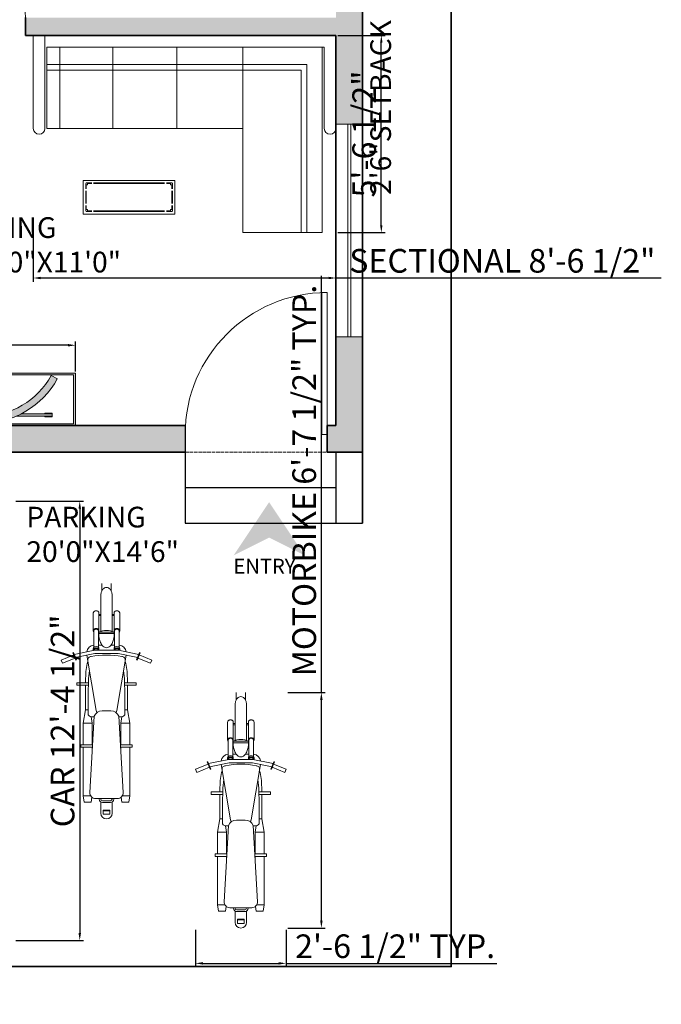
# Model space of a CAD drawing. Units: inches. Extents: x 4732 to 5926, y 2665 to 3255.
# Tile 5 of 8: x 5104 to 5321, y 2723 to 3056. Entities that reach past the tile are written whole.
import ezdxf

# ---------------------------------------------------------------- set-up
doc = ezdxf.new("R2010")
doc.units = ezdxf.units.IN
doc.linetypes.add('ACAD_ISO02W100', pattern=[15, 12, -3])
for name, color, linetype, lineweight in [('A-ANNO-DIMS', 2, 'Continuous', 18), ('A-ANNO-SYMB', 7, 'Continuous', 18), ('A-ANNO-TEXT', 7, 'Continuous', 18), ('A-AREA-IDEN', 7, 'Continuous', 18), ('A-DOOR', 3, 'Continuous', 18), ('A-FLOR-STRS', 7, 'Continuous', 25), ('A-FLOR-STRS-HIDN', 8, 'ACAD_ISO02W100', 18), ('A-GLAZ', 4, 'Continuous', 18), ('A-SITE-VEHS', 8, 'Continuous', 13), ('A-WALL', 7, 'Continuous', 35), ('A-WALL-PATT', 8, 'Continuous', 13), ('aparador', 36, 'Continuous', 9), ('C-PROP', 7, 'Continuous', 35), ('moveis', 254, 'Continuous', 5), ('NOI THAT', 42, 'Continuous', 18)]:
    doc.layers.add(name, color=color, linetype=linetype, lineweight=lineweight)
doc.styles.get("Standard").update_dxf_attribs({"font": 'arial.ttf'})
doc.dimstyles.new('ISO-25', dxfattribs={"dimtxt": 8, "dimasz": 2.5, "dimexe": 1.25, "dimexo": 0.625, "dimtad": 1, "dimdec": 1, "dimlunit": 3, "dimtxsty": 'Standard', "dimcen": 2.5, "dimadec": 0, "dimazin": 0, "dimtfac": 1, "dimtdec": 1, "dimtmove": 0, "dimatfit": 3, "dimfxl": 1, "dimarcsym": 0})

# ---------------------------------------------------------------- blocks, each defined once
blk = doc.blocks.new('TABLE-30A')
at = {"color": 0, "linetype": 'ByBlock'}
for p, q in [((0, 0), (0, 0.55)), ((0, 0.55), (1.5, 0.55)), ((0.051, 0.508), (0.042, 0.499)), ((0.042, 0.499), (0.042, 0.478)), ((0.072, 0.508), (0.051, 0.508)), ((0.072, 0.478), (0.072, 0.508)), ((0.072, 0.508), (0.14, 0.508)), ((0.072, 0.499), (0.14, 0.499)), ((1.331, 0.508), (0.169, 0.508)), ((1.331, 0.499), (0.169, 0.499)), ((1.428, 0.508), (1.36, 0.508)), ((1.428, 0.499), (1.36, 0.499)), ((1.428, 0.508), (1.428, 0.478)), ((1.449, 0.508), (1.428, 0.508)), ((1.458, 0.499), (1.449, 0.508)), ((1.458, 0.478), (1.458, 0.499)), ((1.5, 0.55), (1.5, 0)), ((0.042, 0.478), (0.072, 0.478)), ((0.042, 0.478), (0.042, 0.41)), ((0.042, 0.169), (0.042, 0.381)), ((0.051, 0.478), (0.051, 0.41)), ((0.051, 0.169), (0.051, 0.381)), ((1.428, 0.478), (1.458, 0.478)), ((1.449, 0.478), (1.449, 0.41)), ((1.449, 0.381), (1.449, 0.169)), ((1.458, 0.478), (1.458, 0.41)), ((1.458, 0.381), (1.458, 0.169)), ((1.5, 0), (0, 0)), ((0.042, 0.072), (0.042, 0.14)), ((0.042, 0.072), (0.042, 0.051)), ((0.072, 0.072), (0.042, 0.072)), ((0.042, 0.051), (0.051, 0.042)), ((0.051, 0.072), (0.051, 0.14)), ((0.051, 0.042), (0.072, 0.042)), ((0.072, 0.042), (0.072, 0.072)), ((0.072, 0.051), (0.14, 0.051)), ((0.072, 0.042), (0.14, 0.042)), ((0.169, 0.051), (1.331, 0.051)), ((0.169, 0.042), (1.331, 0.042)), ((1.428, 0.051), (1.36, 0.051)), ((1.428, 0.042), (1.36, 0.042)), ((1.428, 0.072), (1.428, 0.042)), ((1.458, 0.072), (1.428, 0.072)), ((1.428, 0.042), (1.449, 0.042)), ((1.449, 0.072), (1.449, 0.14)), ((1.449, 0.042), (1.458, 0.051)), ((1.458, 0.072), (1.458, 0.14)), ((1.458, 0.051), (1.458, 0.072))]:
    blk.add_line(p, q, dxfattribs=at)
blk = doc.blocks.new('12')
at = {"color": 0}
for p, q in [((5656.26, 3021.25), (5553.9, 3021.25)), ((5553.9, 3021.25), (5553.9, 2989.76)), ((5557.83, 3021.25), (5557.83, 2989.76)), ((5656.26, 2989.76), (5656.26, 3021.25)), ((5652.32, 3017.31), (5558.49, 3017.31)), ((5558.49, 3017.31), (5558.49, 2989.76)), ((5562.89, 3017.31), (5562.89, 2989.76)), ((5580.8, 3017.31), (5580.8, 2989.76)), ((5602.45, 3017.31), (5602.45, 2989.76)), ((5624.76, 3017.31), (5624.76, 2954.53)), ((5651.66, 3017.31), (5651.66, 2954.53)), ((5652.32, 2989.76), (5652.32, 3017.31)), ((5646.42, 3011.41), (5558.49, 3011.41)), ((5646.42, 2954.53), (5646.42, 3011.41)), ((5644.45, 3009.44), (5558.49, 3009.44)), ((5644.45, 2954.53), (5644.45, 3009.44)), ((5624.76, 2995), (5624.76, 2954.53)), ((5558.49, 2989.76), (5624.76, 2989.76)), ((5651.66, 2954.53), (5624.76, 2954.53))]:
    blk.add_line(p, q, dxfattribs=at)
for centre in [(5555.86, 2989.76), (5654.29, 2989.76)]:
    blk.add_arc(centre, 1.97, 180, 0, dxfattribs=at)
at = {"xscale": -20.70834898381633, "yscale": 20.70834898381633, "zscale": 20.70834898381633}
blk.add_blockref('TABLE-30A', (5601.8, 2960.82), dxfattribs=at)
blk = doc.blocks.new('Aparador ORGANICA Formatto')
at = {"layer": 'aparador', "ltscale": 0.3}
h = blk.add_hatch(color=256, dxfattribs=at)
h.dxf.hatch_style = 1
h.set_gradient(color1=(118, 213, 123), color2=(52, 168, 57), one_color=1, tint=0.43, name='INVCURVED')
h.paths.add_polyline_path([(0.8, 0.45), (-0.8, 0.45), (-0.8, 0), (0.8, 0)])
h.paths.add_polyline_path([(0.785, 0.435), (0.785, 0.015), (-0.785, 0.015), (-0.785, 0.435)], flags=16)
h.paths.add_polyline_path([(0.2911, 0.3699), (0.5365, 0.3699), (0.5365, 0.3757), (0.6011, 0.3757), (0.6011, 0.3699), (0.6011, 0.3499), (0.6011, 0.3441), (0.5365, 0.3441), (0.5365, 0.3499), (0.3338, 0.3499, -0.150336), (0.6449, 0.0488), (0.5923, 0.0199, 0.208852), (0.1632, 0.3499), (-0.1632, 0.3499, 0.208852), (-0.5923, 0.0199), (-0.6449, 0.0488, -0.150336), (-0.3338, 0.3499), (-0.5365, 0.3499), (-0.5365, 0.3441), (-0.6011, 0.3441), (-0.6011, 0.3499), (-0.6011, 0.3699), (-0.6011, 0.3757), (-0.5365, 0.3757), (-0.5365, 0.3699), (-0.2911, 0.3699, -0.206106)], flags=0)
h = blk.add_hatch(color=256, dxfattribs=at)
h.dxf.hatch_style = 1
h.set_gradient(color1=(135, 92, 69), color2=(0, 0, 0), one_color=1, name='INVCURVED')
h.paths.add_polyline_path([(-0.6449, 0.0488), (-0.5923, 0.0199, -0.590888), (0.5923, 0.0199), (0.6449, 0.0488, 0.590888)])
h = blk.add_hatch(color=256, dxfattribs=at)
h.dxf.hatch_style = 1
h.set_gradient(color1=(178, 189, 189), one_color=1, tint=1, name='CYLINDER')
h.paths.add_polyline_path([(-0.5365, 0.3757), (-0.6011, 0.3757), (-0.6011, 0.3699), (-0.5365, 0.3699)])
h.paths.add_polyline_path([(-0.5365, 0.3499), (-0.6011, 0.3499), (-0.6011, 0.3441), (-0.5365, 0.3441)])
h = blk.add_hatch(color=256, dxfattribs=at)
h.dxf.hatch_style = 1
h.set_gradient(color1=(118, 213, 123), color2=(31, 101, 35), one_color=1, tint=0.26, name='INVCURVED')
h.paths.add_polyline_path([(-0.2911, 0.3699), (-0.6011, 0.3699), (-0.6011, 0.3499), (-0.3338, 0.3499, -0.015999)])
h = blk.add_hatch(color=256, dxfattribs=at)
h.dxf.hatch_style = 1
h.set_gradient(color1=(118, 213, 123), color2=(31, 101, 35), one_color=1, tint=0.26, name='INVCURVED')
h.paths.add_polyline_path([(-0.1632, 0.3499), (0.1632, 0.3499, 0.122516)])
h = blk.add_hatch(color=256, dxfattribs=at)
h.dxf.hatch_style = 1
h.set_gradient(color1=(118, 213, 123), color2=(31, 101, 35), one_color=1, tint=0.26, name='INVCURVED')
h.paths.add_polyline_path([(0.6011, 0.3699), (0.2911, 0.3699, -0.015999), (0.3338, 0.3499), (0.6011, 0.3499)])
h = blk.add_hatch(color=256, dxfattribs=at)
h.dxf.hatch_style = 1
h.set_gradient(color1=(178, 189, 189), one_color=1, tint=1, name='CYLINDER')
h.paths.add_polyline_path([(0.6011, 0.3757), (0.5365, 0.3757), (0.5365, 0.3699), (0.6011, 0.3699)])
h.paths.add_polyline_path([(0.6011, 0.3499), (0.5365, 0.3499), (0.5365, 0.3441), (0.6011, 0.3441)])
for p, q in [((-0.5923, 0.0199), (-0.6449, 0.0488)), ((0.5923, 0.0199), (0.6449, 0.0488))]:
    blk.add_line(p, q, dxfattribs=at)
for points in [[(-0.6011, 0.3699), (-0.6011, 0.3757), (-0.5365, 0.3757), (-0.5365, 0.3699)], [(-0.5365, 0.3499), (-0.5365, 0.3441), (-0.6011, 0.3441), (-0.6011, 0.3499)], [(0.6011, 0.3699), (0.6011, 0.3757), (0.5365, 0.3757), (0.5365, 0.3699)], [(0.5365, 0.3499), (0.5365, 0.3441), (0.6011, 0.3441), (0.6011, 0.3499)]]:
    blk.add_lwpolyline(points, dxfattribs=at)
for radius in [0.7362, 0.6762]:
    blk.add_arc((0, -0.3063), radius, 28.84335, 151.15665, dxfattribs=at)
at = {"layer": 'moveis', "ltscale": 0.3}
for p, q in [((-0.6011, 0.3699), (-0.6011, 0.3499)), ((-0.2911, 0.3699), (-0.6011, 0.3699)), ((-0.6011, 0.3499), (-0.3338, 0.3499)), ((-0.1632, 0.3499), (0.1632, 0.3499)), ((0.2911, 0.3699), (0.6011, 0.3699)), ((0.6011, 0.3499), (0.3338, 0.3499)), ((0.6011, 0.3699), (0.6011, 0.3499))]:
    blk.add_line(p, q, dxfattribs=at)
for points in [[(-0.8, 0), (0.8, 0), (0.8, 0.45), (-0.8, 0.45)], [(-0.785, 0.015), (0.785, 0.015), (0.785, 0.435), (-0.785, 0.435)]]:
    blk.add_lwpolyline(points, close=True, dxfattribs=at)
blk = doc.blocks.new('*U20')
for p, q in [((0, 0), (0, -6)), ((36, 0), (36, -6))]:
    blk.add_line(p, q)
blk.add_lwpolyline([(0, 0), (0, 36), (1.75, 36), (1.75, 0)], close=True)
blk.add_arc((0, 0), 36, 0, 90)
blk = doc.blocks.new('BIKE')
for p, q in [((34846.04, 15170.34), (34846.04, 15168.87)), ((34847.86, 15170.34), (34847.86, 15168.87)), ((34845.81, 15167.86), (34845.81, 15160.7)), ((34845.81, 15167.86), (34845.81, 15160.7)), ((34848.09, 15167.86), (34848.09, 15160.7)), ((34844.29, 15164.4), (34844.29, 15160.81)), ((34845.43, 15164.4), (34845.43, 15160.81)), ((34845.43, 15164.1), (34845.81, 15164.1)), ((34845.43, 15163.85), (34845.81, 15163.85)), ((34848.47, 15164.1), (34848.09, 15164.1)), ((34848.47, 15163.85), (34848.09, 15163.85)), ((34848.47, 15164.4), (34848.47, 15160.81)), ((34849.61, 15164.4), (34849.61, 15160.81)), ((34844.41, 15160.81), (34844.41, 15157.43)), ((34845.32, 15160.81), (34845.32, 15157.43)), ((34848.51, 15160.53), (34845.39, 15160.53)), ((34845.39, 15160.23), (34845.39, 15160.53)), ((34845.39, 15160.23), (34845.39, 15160.53)), ((34848.51, 15160.23), (34845.39, 15160.23)), ((34848.51, 15160.23), (34848.51, 15160.53)), ((34848.58, 15160.81), (34848.58, 15157.43)), ((34849.5, 15160.81), (34849.5, 15157.43)), ((34845.32, 15157.92), (34846.04, 15157.92)), ((34848.58, 15157.92), (34847.87, 15157.92)), ((34837.84, 15154.89), (34840.37, 15155.93)), ((34840.19, 15156.35), (34840.3, 15156.39)), ((34840.19, 15156.35), (34840.8, 15154.88)), ((34840.3, 15156.39), (34840.9, 15154.92)), ((34840.47, 15155.97), (34840.8, 15156.11)), ((34840.8, 15156.11), (34844.56, 15156.88)), ((34841, 15155.45), (34844.63, 15156.2)), ((34844.86, 15144.72), (34843.01, 15155.87)), ((34844.29, 15156.87), (34844.29, 15157.17)), ((34844.41, 15156.87), (34844.41, 15156.85)), ((34844.56, 15156.88), (34846.95, 15156.88)), ((34844.63, 15156.2), (34846.95, 15156.2)), ((34845.43, 15156.87), (34845.43, 15157.17)), ((34849.34, 15156.88), (34846.95, 15156.88)), ((34849.27, 15156.2), (34846.95, 15156.2)), ((34848.47, 15156.87), (34848.47, 15157.17)), ((34849.05, 15144.72), (34850.89, 15155.87)), ((34852.9, 15155.45), (34849.27, 15156.2)), ((34853.1, 15156.11), (34849.34, 15156.88)), ((34849.5, 15156.87), (34849.5, 15156.85)), ((34849.61, 15156.87), (34849.61, 15157.17)), ((34853.6, 15156.39), (34853, 15154.92)), ((34853.71, 15156.35), (34853.1, 15154.88)), ((34853.43, 15155.97), (34853.1, 15156.11)), ((34856.07, 15154.89), (34853.54, 15155.93)), ((34853.71, 15156.35), (34853.6, 15156.39)), ((34837.84, 15154.89), (34838.1, 15154.26)), ((34838.1, 15154.26), (34840.63, 15155.3)), ((34840.73, 15155.34), (34841, 15155.45)), ((34840.8, 15154.88), (34840.9, 15154.92)), ((34842.8, 15152.59), (34843.06, 15154.2)), ((34843.06, 15154.2), (34843.22, 15154.58)), ((34850.84, 15154.2), (34850.68, 15154.58)), ((34851.1, 15152.59), (34850.84, 15154.2)), ((34853.17, 15155.34), (34852.9, 15155.45)), ((34853.1, 15154.88), (34853, 15154.92)), ((34855.81, 15154.26), (34853.28, 15155.3)), ((34856.07, 15154.89), (34855.81, 15154.26)), ((34842.7, 15150.31), (34842.8, 15152.59)), ((34843.33, 15151.09), (34843.52, 15152.8)), ((34850.57, 15151.09), (34850.38, 15152.8)), ((34851.2, 15150.31), (34851.1, 15152.59)), ((34840.97, 15150.31), (34843.3, 15150.31)), ((34840.97, 15149.81), (34840.97, 15150.31)), ((34843.29, 15149.81), (34840.97, 15149.81)), ((34842.7, 15144.87), (34842.7, 15149.81)), ((34843.23, 15147.75), (34843.33, 15151.09)), ((34850.67, 15147.75), (34850.57, 15151.09)), ((34852.93, 15150.31), (34850.6, 15150.31)), ((34850.61, 15149.81), (34852.93, 15149.81)), ((34851.2, 15144.87), (34851.2, 15149.81)), ((34852.93, 15149.81), (34852.93, 15150.31)), ((34843.23, 15144.15), (34843.23, 15147.75)), ((34850.67, 15144.15), (34850.67, 15147.75)), ((34842.7, 15144.87), (34842.25, 15142.19)), ((34842.7, 15144.87), (34843.23, 15144.87)), ((34847.85, 15144.64), (34846.06, 15144.64)), ((34851.2, 15144.87), (34850.67, 15144.87)), ((34851.2, 15144.87), (34851.65, 15142.19)), ((34842.25, 15142.19), (34844.07, 15142.19)), ((34842.25, 15137.82), (34842.25, 15142.19)), ((34844.46, 15143.56), (34843.6, 15128.2)), ((34843.85, 15143.46), (34844.07, 15142.19)), ((34843.91, 15143.46), (34844.46, 15143.46)), ((34844.07, 15137.82), (34844.07, 15142.19)), ((34849.44, 15143.56), (34850.3, 15128.2)), ((34849.99, 15143.46), (34849.44, 15143.46)), ((34850.05, 15143.46), (34849.83, 15142.19)), ((34851.65, 15142.19), (34849.83, 15142.19)), ((34849.83, 15137.82), (34849.83, 15142.19)), ((34851.65, 15137.82), (34851.65, 15142.19)), ((34841.79, 15137.82), (34844.14, 15137.82)), ((34841.79, 15137.33), (34841.79, 15137.82)), ((34844.11, 15137.33), (34841.79, 15137.33)), ((34842.25, 15127.57), (34842.25, 15137.33)), ((34844.07, 15136.55), (34844.07, 15137.33)), ((34852.11, 15137.82), (34849.76, 15137.82)), ((34849.79, 15137.33), (34852.11, 15137.33)), ((34849.83, 15136.55), (34849.83, 15137.33)), ((34851.65, 15127.57), (34851.65, 15137.33)), ((34852.11, 15137.33), (34852.11, 15137.82)), ((34842.25, 15127.57), (34843.75, 15127.57)), ((34842.25, 15127.57), (34842.48, 15126.27)), ((34842.48, 15126.27), (34843.84, 15126.27)), ((34844.02, 15127.25), (34843.84, 15126.27)), ((34849.16, 15126.99), (34844.74, 15126.99)), ((34845.47, 15126.99), (34845.47, 15126.88)), ((34845.81, 15126.99), (34845.81, 15126.88)), ((34845.81, 15126.29), (34845.81, 15124.03)), ((34847.75, 15126.54), (34846.15, 15126.54)), ((34847.75, 15126.2), (34846.15, 15126.2)), ((34848.09, 15126.99), (34848.09, 15126.88)), ((34848.09, 15126.29), (34848.09, 15124.03)), ((34848.43, 15126.99), (34848.43, 15126.88)), ((34849.89, 15127.25), (34850.06, 15126.27)), ((34851.43, 15126.27), (34850.06, 15126.27)), ((34851.65, 15127.57), (34850.15, 15127.57)), ((34851.65, 15127.57), (34851.43, 15126.27)), ((34846.29, 15123.82), (34846.29, 15124.66)), ((34846.29, 15124.66), (34847.61, 15124.66)), ((34846.29, 15124.55), (34847.61, 15124.55)), ((34847.61, 15124.66), (34847.61, 15123.82)), ((34847.61, 15123.82), (34846.29, 15123.82))]:
    blk.add_line(p, q)
for points in [[(34845.81, 15167.86, -0.068977), (34845.9, 15168.53, -0.081012), (34846.15, 15169.05, -0.107014), (34846.54, 15169.42, -0.137239), (34846.95, 15169.53, -0.137239), (34847.36, 15169.42, -0.107014), (34847.76, 15169.05, -0.081012), (34848, 15168.53, -0.068977), (34848.09, 15167.86, -0.068977)], [(34845.43, 15164.4, 0.125099), (34845.39, 15164.56, 0.105827), (34845.27, 15164.71, 0.086577), (34845.09, 15164.8, 0.0766), (34844.86, 15164.84, 0.0766), (34844.64, 15164.8, 0.086577), (34844.46, 15164.71, 0.105827), (34844.33, 15164.56, 0.125099), (34844.29, 15164.4, 0.125099)], [(34848.47, 15164.4, -0.125099), (34848.51, 15164.56, -0.105827), (34848.64, 15164.71, -0.086577), (34848.82, 15164.8, -0.0766), (34849.04, 15164.84, -0.0766), (34849.26, 15164.8, -0.086577), (34849.44, 15164.71, -0.105827), (34849.57, 15164.56, -0.125099), (34849.61, 15164.4, -0.125099)], [(34845.32, 15160.55, 0.067261), (34845.39, 15160.65, 0.125099), (34845.43, 15160.81, 0.125099), (34845.39, 15160.97, 0.105827), (34845.27, 15161.12, 0.086577), (34845.09, 15161.21, 0.0766), (34844.86, 15161.25, 0.0766), (34844.64, 15161.21, 0.086577), (34844.46, 15161.12, 0.105827), (34844.33, 15160.97, 0.125099), (34844.29, 15160.81, 0.125099)], [(34844.29, 15160.81, 0.125099), (34844.33, 15160.65, 0.067261), (34844.41, 15160.55, 0.086577)], [(34845.32, 15160.81, 0.125099), (34845.29, 15160.92, 0.105827), (34845.2, 15161.03, 0.086577), (34845.05, 15161.1, 0.0766), (34844.86, 15161.13, 0.0766), (34844.67, 15161.1, 0.086577), (34844.53, 15161.03, 0.105827), (34844.43, 15160.92, 0.125099), (34844.41, 15160.81, 0.125099)], [(34846.95, 15157.37, -0.163989), (34846.41, 15157.55, -0.105862), (34845.85, 15158.21, -0.069323), (34845.52, 15159.08, -0.055531), (34845.39, 15160.23, -0.055531)], [(34848.51, 15160.23, -0.055531), (34848.38, 15159.08, -0.069323), (34848.06, 15158.21, -0.105862), (34847.49, 15157.55, -0.163989), (34846.95, 15157.37, -0.163989)], [(34848.58, 15160.55, -0.067261), (34848.51, 15160.65, -0.125099), (34848.47, 15160.81, -0.125099), (34848.51, 15160.97, -0.105827), (34848.64, 15161.12, -0.086577), (34848.82, 15161.21, -0.0766), (34849.04, 15161.25, -0.0766), (34849.26, 15161.21, -0.086577), (34849.44, 15161.12, -0.105827), (34849.57, 15160.97, -0.125099), (34849.61, 15160.81, -0.125099)], [(34848.58, 15160.81, -0.125099), (34848.61, 15160.92, -0.105827), (34848.71, 15161.03, -0.086577), (34848.85, 15161.1, -0.0766), (34849.04, 15161.13, -0.0766), (34849.23, 15161.1, -0.086577), (34849.37, 15161.03, -0.105827), (34849.47, 15160.92, -0.125099), (34849.5, 15160.81, -0.125099)], [(34849.61, 15160.81, -0.125099), (34849.57, 15160.65, -0.067261), (34849.5, 15160.55, -0.086577)], [(34845.43, 15157.17, 0.125099), (34845.39, 15157.33, 0.105827), (34845.27, 15157.48, 0.086577), (34845.09, 15157.57, 0.0766), (34844.86, 15157.6, 0.0766), (34844.64, 15157.57, 0.086577), (34844.46, 15157.48, 0.105827), (34844.33, 15157.33, 0.125099), (34844.29, 15157.17, 0.125099)], [(34845.43, 15156.88, 0.117252), (34845.39, 15157.03, 0.105827), (34845.27, 15157.18, 0.086577), (34845.09, 15157.27, 0.0766), (34844.86, 15157.31, 0.0766), (34844.64, 15157.27, 0.086577), (34844.46, 15157.18, 0.105827), (34844.33, 15157.03, 0.125099), (34844.29, 15156.87, 0.125099)], [(34844.29, 15156.87, 0.032819), (34844.3, 15156.83, 0.067261)], [(34845.32, 15156.88, 0.113202), (34845.29, 15156.98, 0.105827), (34845.2, 15157.09, 0.086577), (34845.05, 15157.16, 0.0766), (34844.86, 15157.19, 0.0766), (34844.67, 15157.16, 0.086577), (34844.53, 15157.09, 0.105827), (34844.43, 15156.98, 0.125099), (34844.41, 15156.87, 0.125099)], [(34848.47, 15157.17, -0.125099), (34848.51, 15157.33, -0.105827), (34848.64, 15157.48, -0.086577), (34848.82, 15157.57, -0.0766), (34849.04, 15157.6, -0.0766), (34849.26, 15157.57, -0.086577), (34849.44, 15157.48, -0.105827), (34849.57, 15157.33, -0.125099), (34849.61, 15157.17, -0.125099)], [(34848.47, 15156.88, -0.117252), (34848.51, 15157.03, -0.105827), (34848.64, 15157.18, -0.086577), (34848.82, 15157.27, -0.0766), (34849.04, 15157.31, -0.0766), (34849.26, 15157.27, -0.086577), (34849.44, 15157.18, -0.105827), (34849.57, 15157.03, -0.125099), (34849.61, 15156.87, -0.125099)], [(34848.58, 15156.88, -0.113202), (34848.61, 15156.98, -0.105827), (34848.71, 15157.09, -0.086577), (34848.85, 15157.16, -0.0766), (34849.04, 15157.19, -0.0766), (34849.23, 15157.16, -0.086577), (34849.37, 15157.09, -0.105827), (34849.47, 15156.98, -0.125099), (34849.5, 15156.87, -0.125099)], [(34849.61, 15156.87, -0.032819), (34849.61, 15156.83, -0.067261)]]:
    blk.add_lwpolyline(points, format="xyb")
for centre, radius, start, end in [((34846.95, 15157.24), 3.64, 64.5882, 115.4118), ((34844.55, 15156.32), 1.59, 95.2207, 171.678), ((34849.35, 15156.32), 1.59, 8.322, 84.7793), ((34846.95, 15140.12), 15.79, 78.7129, 101.2871), ((34843.86, 15154.92), 0.684, 90, 189.3898), ((34850.04, 15154.92), 0.684, 350.6102, 90), ((34843.91, 15144.15), 0.684, 180, 270), ((34846, 15143), 1.64, 88.1125, 159.9264), ((34845.53, 15144.83), 0.684, 189.3898, 226.4877), ((34847.9, 15143), 1.64, 20.0736, 91.8875), ((34848.37, 15144.83), 0.684, 313.5123, 350.6102), ((34849.99, 15144.15), 0.684, 270, 0), ((34844.74, 15128.13), 1.14, 176.7865, 270), ((34849.16, 15128.13), 1.14, 270, 3.2135), ((34846.15, 15126.88), 0.684, 180, 270), ((34846.15, 15126.88), 0.342, 180, 270), ((34847.75, 15126.88), 0.684, 270, 0), ((34847.75, 15126.88), 0.342, 270, 0), ((34846.95, 15124.03), 1.14, 180, 0)]:
    blk.add_arc(centre, radius, start, end)
blk = doc.blocks.new('GLAZ-UNIT-72IN')
for p, q in [((0, 72), (0, 0)), ((1, 72), (1, 0))]:
    blk.add_line(p, q)
blk = doc.blocks.new('*D80')
at = {"layer": 'A-ANNO-DIMS', "color": 0, "lineweight": -2, "transparency": 16777216}
for p, q in [((5206.46, 2828.61), (5206.46, 2969.57)), ((5195.13, 2828.61), (5207.71, 2828.61)), ((5206.46, 2751.44), (5206.46, 2826.11)), ((5195.13, 2748.94), (5207.71, 2748.94))]:
    blk.add_line(p, q, dxfattribs=at)
at = {"layer": 'A-ANNO-DIMS', "color": 0, "transparency": 16777216}
for points in [[(5206.04, 2826.11), (5206.87, 2826.11), (5206.46, 2828.61)], [(5206.04, 2751.44), (5206.87, 2751.44), (5206.46, 2748.94)]]:
    blk.add_solid(points, dxfattribs=at)
at = {"layer": 'Defpoints', "color": 0, "transparency": 16777216}
for p in [(5194.51, 2828.61), (5206.46, 2828.61), (5194.51, 2748.94)]:
    blk.add_point(p, dxfattribs=at)
at = {"layer": 'A-ANNO-DIMS', "color": 0, "transparency": 16777216, "insert": (5201.69, 2900.34), "char_height": 8, "attachment_point": 5, "rotation": 90}
blk.add_mtext('MOTORBIKE 6\'-7 1/2" TYP.', dxfattribs=at)
blk = doc.blocks.new('*D81')
at = {"layer": 'A-ANNO-DIMS', "color": 0, "lineweight": -2, "transparency": 16777216}
for p, q in [((5163.91, 2748.32), (5163.91, 2735.74)), ((5194.51, 2748.32), (5194.51, 2735.74)), ((5166.41, 2736.99), (5192.01, 2736.99)), ((5194.51, 2736.99), (5265.8, 2736.99))]:
    blk.add_line(p, q, dxfattribs=at)
at = {"layer": 'A-ANNO-DIMS', "color": 0, "transparency": 16777216}
for points in [[(5166.41, 2737.41), (5166.41, 2736.57), (5163.91, 2736.99)], [(5192.01, 2737.41), (5192.01, 2736.57), (5194.51, 2736.99)]]:
    blk.add_solid(points, dxfattribs=at)
at = {"layer": 'Defpoints', "color": 0, "transparency": 16777216}
for p in [(5163.91, 2748.94), (5194.51, 2748.94), (5194.51, 2736.99)]:
    blk.add_point(p, dxfattribs=at)
at = {"layer": 'A-ANNO-DIMS', "color": 0, "transparency": 16777216, "insert": (5231.4, 2741.75), "char_height": 8, "attachment_point": 5}
blk.add_mtext('2\'-6 1/2" TYP.', dxfattribs=at)
blk = doc.blocks.new('*D92')
at = {"layer": 'A-ANNO-DIMS', "color": 0, "lineweight": -2, "transparency": 16777216}
for p, q in [((5109.02, 2983.58), (5109.02, 2967.6)), ((5211.38, 2983.58), (5211.38, 2967.6)), ((5111.52, 2968.85), (5208.88, 2968.85)), ((5211.38, 2968.85), (5321.45, 2968.85))]:
    blk.add_line(p, q, dxfattribs=at)
at = {"layer": 'A-ANNO-DIMS', "color": 0, "transparency": 16777216}
for points in [[(5111.52, 2969.27), (5111.52, 2968.44), (5109.02, 2968.85)], [(5208.88, 2969.27), (5208.88, 2968.44), (5211.38, 2968.85)]]:
    blk.add_solid(points, dxfattribs=at)
at = {"layer": 'Defpoints', "color": 0, "transparency": 16777216}
for p in [(5109.02, 2984.21), (5211.38, 2984.21), (5211.38, 2968.85)]:
    blk.add_point(p, dxfattribs=at)
at = {"layer": 'A-ANNO-DIMS', "color": 0, "transparency": 16777216, "insert": (5267.67, 2973.62), "char_height": 8, "attachment_point": 5}
blk.add_mtext('SECTIONAL 8\'-6 1/2"', dxfattribs=at)
blk = doc.blocks.new('*D93')
at = {"layer": 'A-ANNO-DIMS', "color": 0, "lineweight": -2, "transparency": 16777216}
for p, q in [((5212.01, 3050.93), (5227.99, 3050.93)), ((5226.74, 2986.71), (5226.74, 3048.43)), ((5212.01, 2984.21), (5227.99, 2984.21))]:
    blk.add_line(p, q, dxfattribs=at)
at = {"layer": 'A-ANNO-DIMS', "color": 0, "transparency": 16777216}
for points in [[(5226.32, 3048.43), (5227.15, 3048.43), (5226.74, 3050.93)], [(5226.32, 2986.71), (5227.15, 2986.71), (5226.74, 2984.21)]]:
    blk.add_solid(points, dxfattribs=at)
at = {"layer": 'Defpoints', "color": 0, "transparency": 16777216}
for p in [(5211.38, 3050.93), (5226.74, 3050.93), (5211.38, 2984.21)]:
    blk.add_point(p, dxfattribs=at)
at = {"layer": 'A-ANNO-DIMS', "color": 0, "transparency": 16777216, "insert": (5221.97, 3017.57), "char_height": 8, "attachment_point": 5, "rotation": 90}
blk.add_mtext('5\'-6 1/2"', dxfattribs=at)
blk = doc.blocks.new('*D94')
at = {"layer": 'A-ANNO-DIMS', "color": 0, "lineweight": -2, "transparency": 16777216}
for p, q in [((5060.26, 2946.1), (4966.35, 2946.1)), ((5060.26, 2937.27), (5060.26, 2947.35)), ((5120.75, 2946.1), (5062.76, 2946.1)), ((5123.25, 2937.27), (5123.25, 2947.35))]:
    blk.add_line(p, q, dxfattribs=at)
at = {"layer": 'A-ANNO-DIMS', "color": 0, "transparency": 16777216}
for points in [[(5062.76, 2946.52), (5062.76, 2945.68), (5060.26, 2946.1)], [(5120.75, 2946.52), (5120.75, 2945.68), (5123.25, 2946.1)]]:
    blk.add_solid(points, dxfattribs=at)
at = {"layer": 'Defpoints', "color": 0, "transparency": 16777216}
for p in [(5060.26, 2946.1), (5060.26, 2936.65), (5123.25, 2936.65)]:
    blk.add_point(p, dxfattribs=at)
at = {"layer": 'A-ANNO-DIMS', "color": 0, "transparency": 16777216, "insert": (5012.05, 2950.87), "char_height": 8, "attachment_point": 5}
blk.add_mtext('SIDEBOARD 5\'-3"', dxfattribs=at)
blk = doc.blocks.new('*D96')
at = {"layer": 'A-ANNO-DIMS', "color": 0, "lineweight": -2, "transparency": 16777216}
for p, q in [((5103.06, 2893.31), (5125.97, 2893.31)), ((5124.72, 2890.81), (5124.72, 2747.23)), ((5103.06, 2744.73), (5125.97, 2744.73))]:
    blk.add_line(p, q, dxfattribs=at)
at = {"layer": 'A-ANNO-DIMS', "color": 0, "transparency": 16777216}
for points in [[(5124.3, 2890.81), (5125.14, 2890.81), (5124.72, 2893.31)], [(5124.3, 2747.23), (5125.14, 2747.23), (5124.72, 2744.73)]]:
    blk.add_solid(points, dxfattribs=at)
at = {"layer": 'Defpoints', "color": 0, "transparency": 16777216}
for p in [(5102.43, 2893.31), (5102.43, 2744.73), (5124.72, 2744.73)]:
    blk.add_point(p, dxfattribs=at)
at = {"layer": 'A-ANNO-DIMS', "color": 0, "transparency": 16777216, "insert": (5119.96, 2819.02), "char_height": 8, "attachment_point": 5, "rotation": 90}
blk.add_mtext('CAR 12\'-4 1/2"', dxfattribs=at)

msp = doc.modelspace()

# ---------------------------------------------------------------- hatches: boundary and pattern name
at = {"layer": 'A-ANNO-SYMB'}
h = msp.add_hatch(color=256, dxfattribs=at)
h.dxf.hatch_style = 1
h.paths.add_polyline_path([(5188.79, 2881.01), (5200.79, 2875.01), (5188.79, 2893.01), (5176.79, 2875.01)])
at = {"layer": 'A-WALL-PATT'}
h = msp.add_hatch(color=256, dxfattribs=at)
h.dxf.hatch_style = 1
h.paths.add_polyline_path([(4905.38, 3185.93), (4848.38, 3185.93), (4848.38, 3146.93), (4857.38, 3146.93), (4857.38, 3176.93), (4905.38, 3176.93)])
h.paths.add_polyline_path([(5022.38, 3185.93), (4953.38, 3185.93), (4953.38, 3176.93), (4966.1, 3176.93), (5001.38, 3176.93), (5001.38, 3098.93), (5028.38, 3098.93), (5028.38, 3104.93), (5007.38, 3104.93), (5007.38, 3176.93), (5022.38, 3176.93)])
h.paths.add_polyline_path([(5115.38, 3185.93), (5046.38, 3185.93), (5046.38, 3176.93), (5061.38, 3176.93), (5061.38, 3104.93), (5058.38, 3104.93), (5058.38, 3098.93), (5067.38, 3098.93), (5067.38, 3176.93), (5115.38, 3176.93)])
h.paths.add_polyline_path([(5220.38, 3185.93), (5163.38, 3185.93), (5163.38, 3176.93), (5168.97, 3176.93), (5211.38, 3176.93), (5211.38, 3146.93), (5220.38, 3146.93)])
h.paths.add_polyline_path([(4857.38, 3086.93), (4848.38, 3086.93), (4848.38, 3026.93), (4857.38, 3026.93), (4857.38, 3050.93), (5001.38, 3050.93), (5001.38, 3008.93), (5007.38, 3008.93), (5007.38, 3050.93), (5022.38, 3050.93), (5022.38, 3056.93), (4857.38, 3056.93)])
h.paths.add_polyline_path([(4857.38, 2978.93), (4848.38, 2978.93), (4848.38, 2945.93), (4872.38, 2945.93), (4872.38, 2933.93), (4875.38, 2933.93), (4881.38, 2933.93), (4881.38, 2954.93), (4857.38, 2954.93)])
h.paths.add_polyline_path([(4881.38, 2903.93), (4875.38, 2903.93), (4872.38, 2903.93), (4872.38, 2897.93), (4881.38, 2897.93)])
h.paths.add_polyline_path([(4881.38, 2849.93), (4872.38, 2849.93), (4872.38, 2828.75), (4872.38, 2825.93), (4848.38, 2825.93), (4848.38, 2804.93), (4857.38, 2804.93), (4857.38, 2816.93), (4929.38, 2816.93), (4929.38, 2825.93), (4881.38, 2825.93)])
h.paths.add_polyline_path([(4975.38, 2744.93), (4857.38, 2744.93), (4857.38, 2756.93), (4848.38, 2756.93), (4848.38, 2735.93), (4975.38, 2735.93)])
h.paths.add_polyline_path([(5160.38, 2915.93), (5160.38, 2918.93), (5007.38, 2918.93), (5007.38, 2960.93), (5001.38, 2960.93), (5001.38, 2825.93), (4977.38, 2825.93), (4977.38, 2816.93), (5010.38, 2816.93), (5010.38, 2909.93), (5160.38, 2909.93)])
h.paths.add_polyline_path([(5220.38, 2948.93), (5211.38, 2948.93), (5211.38, 2918.93), (5208.38, 2918.93), (5208.38, 2909.93), (5220.38, 2909.93)])
h.paths.add_polyline_path([(5220.38, 3086.93), (5211.38, 3086.93), (5211.38, 3056.93), (5106.38, 3056.93), (5106.38, 3050.93), (5211.38, 3050.93), (5211.38, 3020.93), (5220.38, 3020.93)])
h.paths.add_polyline_path([(5067.38, 3098.93), (5061.38, 3098.93), (5061.38, 3056.93), (5058.38, 3056.93), (5058.38, 3050.93), (5061.38, 3050.93), (5070.38, 3050.93), (5070.38, 3056.93), (5067.38, 3056.93)])
h.paths.add_polyline_path([(4883.76, 2941.13), (4938.24, 2941.13), (4938.24, 2949.38), (4883.76, 2949.38)], flags=9)
h.paths.add_polyline_path([(4840.48, 3026.79), (4840.48, 3093.88), (4825.54, 3093.88), (4825.54, 3026.79)], flags=9)
h.paths.add_polyline_path([(5245.66, 2994.98), (5245.66, 3062.07), (5230.72, 3062.07), (5230.72, 2994.98)], flags=9)
h.paths.add_polyline_path([(4994.89, 3193.24), (5061.99, 3193.24), (5061.99, 3208.18), (4994.89, 3208.18)], flags=9)
h.paths.add_polyline_path([(5081.53, 3115.35), (5081.53, 3161.13), (5073.28, 3161.13), (5073.28, 3115.35)], flags=25)
h.paths.add_polyline_path([(4997.53, 3115.35), (4997.53, 3161.13), (4989.28, 3161.13), (4989.28, 3115.35)], flags=25)
h.paths.add_polyline_path([(5175.31, 2866.04), (5202.42, 2866.04), (5202.42, 2876.71), (5175.31, 2876.71)], flags=9)
h.paths.add_polyline_path([(4820.13, 2876.28), (4869.1, 2876.28), (4869.1, 2902.89), (4820.13, 2902.89)], flags=9)
h.paths.add_polyline_path([(5104.69, 2868.81), (5158.82, 2868.81), (5158.82, 2895.42), (5104.69, 2895.42)], flags=25)
h.paths.add_polyline_path([(5084.11, 2966.75), (5138.25, 2966.75), (5138.25, 2993.36), (5084.11, 2993.36)], flags=9)
h.paths.add_polyline_path([(4897.84, 3000.24), (4946.81, 3000.24), (4946.81, 3026.85), (4897.84, 3026.85)], flags=9)
h.paths.add_polyline_path([(5009.53, 3133.48), (5059.32, 3133.48), (5059.32, 3160.09), (5009.53, 3160.09)], flags=9)
h.paths.add_polyline_path([(5124.24, 3088.37), (5180.47, 3088.37), (5180.47, 3114.99), (5124.24, 3114.99)], flags=9)
h.paths.add_polyline_path([(4897.52, 3088.37), (4965.52, 3088.37), (4965.52, 3114.99), (4897.52, 3114.99)], flags=9)
h.paths.add_polyline_path([(4924.5, 2879.19), (4978.63, 2879.19), (4978.63, 2905.8), (4924.5, 2905.8)], flags=9)

# ---------------------------------------------------------------- linework, layer by layer
at = {"layer": 'A-DOOR'}
for p, q in [((5160.38, 2915.93), (5160.38, 2909.93)), ((5208.38, 2915.93), (5208.38, 2909.93))]:
    msp.add_line(p, q, dxfattribs=at)
msp.add_lwpolyline([(5208.38, 2915.93), (5208.38, 2963.93), (5206.63, 2963.93), (5206.63, 2915.93)], close=True, dxfattribs=at)
msp.add_arc((5208.38, 2915.93), 48, 90, 180, dxfattribs=at)
at = {"layer": 'A-FLOR-STRS'}
for p, q in [((5160.38, 2918.93), (5160.38, 2885.93)), ((5211.38, 2909.93), (5211.38, 2885.93)), ((5160.38, 2897.93), (5211.38, 2897.93)), ((5160.38, 2885.93), (5220.38, 2885.93))]:
    msp.add_line(p, q, dxfattribs=at)
at = {"layer": 'A-FLOR-STRS-HIDN', "ltscale": 0.1}
msp.add_line((5160.38, 2909.93), (5208.38, 2909.93), dxfattribs=at)
at = {"layer": 'A-GLAZ'}
for p, q in [((5211.38, 3020.93), (5220.38, 3020.93)), ((5211.38, 2948.93), (5220.38, 2948.93))]:
    msp.add_line(p, q, dxfattribs=at)
at = {"layer": 'A-WALL'}
for p, q in [((5220.38, 3185.93), (5220.38, 2885.93)), ((5106.38, 3056.93), (5106.38, 3050.93)), ((5106.38, 3050.93), (5211.38, 3050.93)), ((5211.38, 3050.93), (5211.38, 2918.93)), ((5007.38, 2918.93), (5160.38, 2918.93)), ((5208.38, 2918.93), (5208.38, 2909.93)), ((5208.38, 2918.93), (5211.38, 2918.93)), ((5010.38, 2909.93), (5160.38, 2909.93)), ((5208.38, 2909.93), (5220.38, 2909.93))]:
    msp.add_line(p, q, dxfattribs=at)
at = {"layer": 'C-PROP'}
msp.add_lwpolyline([(4818.38, 3215.93), (5250.38, 3215.93), (5250.38, 2735.93), (4818.38, 2735.93)], close=True, dxfattribs=at)

# ---------------------------------------------------------------- block references
at = {"layer": 'A-DOOR'}
msp.add_blockref('*U20', (5070.38, 3056.93), dxfattribs=at)
at = {"layer": 'A-GLAZ'}
msp.add_blockref('GLAZ-UNIT-72IN', (5215.38, 2948.93), dxfattribs=at)
at = {"layer": 'A-SITE-VEHS', "xscale": 1.67889555227424, "yscale": 1.67889555227424, "zscale": 1.67889555227424}
for p in [(-53370.62, -22603.89), (-53325.18, -22640.81)]:
    msp.add_blockref('BIKE', p, dxfattribs=at)
at = {"layer": 'NOI THAT'}
msp.add_blockref('12', (-444.88, 29.68), dxfattribs=at)
at = {"layer": 'NOI THAT', "xscale": 39.3701, "yscale": 39.3701, "zscale": 39.3701, "rotation": 180}
msp.add_blockref('Aparador ORGANICA Formatto', (5091.75, 2936.65), dxfattribs=at)

# ---------------------------------------------------------------- texts
at = {"layer": 'A-ANNO-TEXT', "insert": (5223.01, 2996.95), "char_height": 7, "attachment_point": 1, "rotation": 90}
msp.add_mtext_dynamic_manual_height_columns('{\\fTimes New Roman|b0|i0|c0|p18; 2\'6"SETBACK }', width=61.0557, gutter_width=12.5, heights=[0], dxfattribs=at)
at = {"layer": 'A-ANNO-TEXT', "insert": (5176.71, 2873.88), "char_height": 5, "attachment_point": 1}
msp.add_mtext_dynamic_manual_height_columns('{\\fTimes New Roman|b0|i0|c0|p18;ENTRY}', width=196.2607, gutter_width=12.5, heights=[0], dxfattribs=at)
at = {"layer": 'A-AREA-IDEN', "char_height": 7, "attachment_point": 1}
for s, insert in [('{\\fTimes New Roman|b0|i0|c0|p18;LIVING 17\'0"X11\'0"}', (5087.07, 2989.4)), ('{\\fTimes New Roman|b0|i0|c0|p18;PARKING\\P20\'0"X14\'6"}', (5106.66, 2891.46))]:
    msp.add_mtext_dynamic_manual_height_columns(s, width=61.0557, gutter_width=12.5, heights=[0], dxfattribs=dict(at, insert=insert))

# ---------------------------------------------------------------- dimensions: what is measured, and where the dimension line sits
at = {"layer": 'A-ANNO-DIMS'}
dim = msp.add_linear_dim(base=(5226.74, 3050.93), p1=(5211.38, 2984.21), p2=(5211.38, 3050.93), angle=90, dimstyle='ISO-25', override={"dimdec": 1, "dimlfac": 1, "dimrnd": 0, "dimzin": 1, "dimdsep": 46, "dimlunit": 4, "dimfrac": 2}, dxfattribs=at)
dim.commit()
dim.dimension.update_dxf_attribs({"geometry": '*D93', "text_midpoint": (5221.97, 3017.57)})
for base, p1, p2, text, picture, middle in [((5211.38, 2968.85), (5109.02, 2984.21), (5211.38, 2984.21), 'SECTIONAL <>', '*D92', (5267.67, 2973.62)), ((5194.51, 2736.99), (5163.91, 2748.94), (5194.51, 2748.94), '<> TYP.', '*D81', (5231.4, 2741.75))]:
    dim = msp.add_linear_dim(base=base, p1=p1, p2=p2, text=text, dimstyle='ISO-25', override={"dimdec": 1, "dimlfac": 1, "dimrnd": 0, "dimzin": 1, "dimdsep": 46, "dimlunit": 4, "dimfrac": 2}, dxfattribs=at)
    dim.commit()
    dim.dimension.update_dxf_attribs({"geometry": picture, "text_midpoint": middle})
for base, p1, p2, angle, text, picture, middle in [((5206.46, 2828.61), (5194.51, 2748.94), (5194.51, 2828.61), 90, 'MOTORBIKE <> TYP.', '*D80', (5201.69, 2900.34)), ((5060.26, 2946.1), (5123.25, 2936.65), (5060.26, 2936.65), 180, 'SIDEBOARD <>', '*D94', (5012.05, 2950.87)), ((5124.72, 2744.73), (5102.43, 2893.31), (5102.43, 2744.73), 270, 'CAR <>', '*D96', (5119.96, 2819.02))]:
    dim = msp.add_linear_dim(base=base, p1=p1, p2=p2, angle=angle, text=text, dimstyle='ISO-25', override={"dimdec": 1, "dimlfac": 1, "dimrnd": 0, "dimzin": 1, "dimdsep": 46, "dimlunit": 4, "dimfrac": 2}, dxfattribs=at)
    dim.commit()
    dim.dimension.update_dxf_attribs({"geometry": picture, "text_midpoint": middle})

doc.saveas('drawing.dxf')
